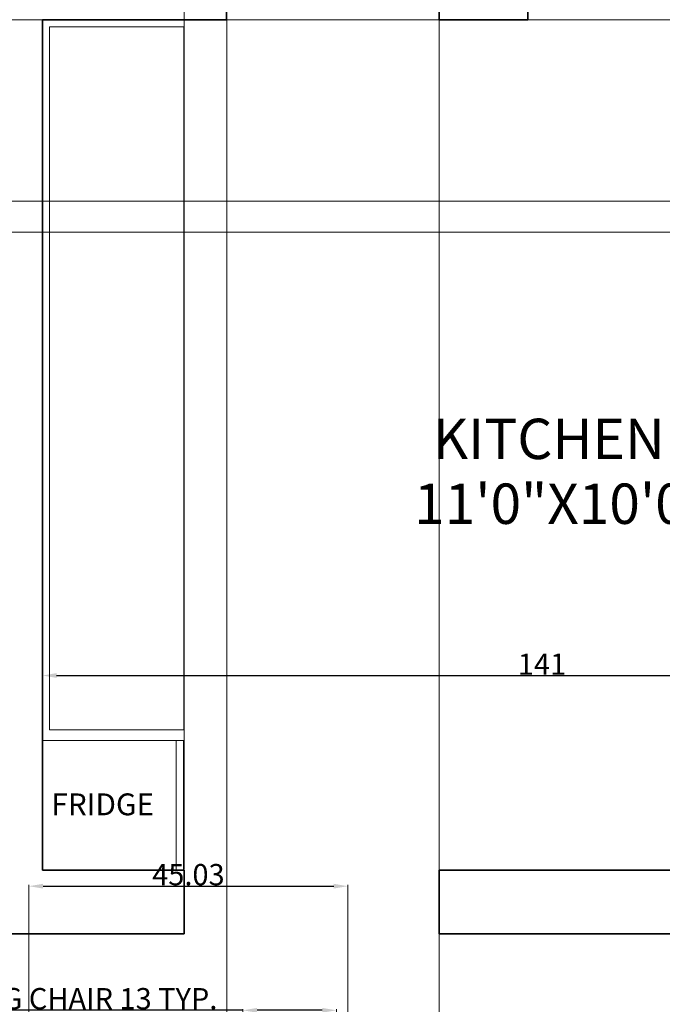
# Model space of a CAD drawing. Units: feet. Extents: x -297 to 770, y -228 to 625.
# Tile 8 of 14: x 589 to 680, y 95 to 233. Entities that reach past the tile are written whole.
import ezdxf

# ---------------------------------------------------------------- set-up
doc = ezdxf.new("R2010")
doc.units = ezdxf.units.FT
doc.header["$MEASUREMENT"] = 0
for name, color, linetype, lineweight in [('A-ANNO-DIMS', 2, 'Continuous', 18), ('A-ANNO-TEXT', 7, 'Continuous', 18), ('A-AREA-IDEN', 7, 'Continuous', 25), ('A-EQPM', 8, 'Continuous', 13), ('A-FLOR-CASE', 8, 'Continuous', 18), ('A-WALL', 7, 'Continuous', 35), ('doors', 30, 'Continuous', 18)]:
    doc.layers.add(name, color=color, linetype=linetype, lineweight=lineweight)
doc.styles.add('Annotative', font='arial.ttf')
doc.styles.get("Standard").update_dxf_attribs({"font": 'arial.ttf'})
doc.dimstyles.get("Standard").update_dxf_attribs({"dimtxt": 3, "dimasz": 2, "dimexe": 0.18, "dimexo": 0.0625, "dimgap": 0.09, "dimtad": 1, "dimtoh": 1, "dimdec": 1, "dimzin": 0, "dimdsep": 46, "dimlunit": 3, "dimtxsty": 'Standard', "dimcen": 0, "dimclre": 256, "dimadec": 0, "dimazin": 0, "dimtfac": 1, "dimtdec": 1, "dimtofl": 0, "dimtmove": 0, "dimatfit": 3, "dimfxl": 1, "dimtolj": 1, "dimtzin": 0, "dimlwe": -1, "dimarcsym": 0})

# ---------------------------------------------------------------- blocks, each defined once
blk = doc.blocks.new('*U6')
for p, q in [((0, 0), (0, -6)), ((40, 0), (40, -6))]:
    blk.add_line(p, q)
blk.add_lwpolyline([(0, 0), (0, 40), (1.75, 40), (1.75, 0)], close=True)
blk.add_arc((0, 0), 40, 0, 90)
blk = doc.blocks.new('*D23')
at = {"layer": 'A-ANNO-DIMS', "color": 0, "lineweight": -2, "transparency": 16777216}
for p, q in [((620.45, 93.67), (573.78, 93.67)), ((631.66, 93.67), (622.45, 93.67))]:
    blk.add_line(p, q, dxfattribs=at)
at = {"layer": 'A-ANNO-DIMS', "transparency": 16777216}
for p, q in [((620.45, 91.75), (620.45, 93.85)), ((633.66, 91.75), (633.66, 93.85))]:
    blk.add_line(p, q, dxfattribs=at)
at = {"layer": 'A-ANNO-DIMS', "color": 0, "transparency": 16777216}
for points in [[(622.45, 94), (622.45, 93.33), (620.45, 93.67)], [(631.66, 94), (631.66, 93.33), (633.66, 93.67)]]:
    blk.add_solid(points, dxfattribs=at)
at = {"layer": 'Defpoints', "color": 0, "transparency": 16777216}
for p in [(620.45, 93.67), (620.45, 91.69), (633.66, 91.69)]:
    blk.add_point(p, dxfattribs=at)
at = {"layer": 'A-ANNO-DIMS', "color": 0, "transparency": 16777216, "insert": (596.11, 95.31), "char_height": 3, "attachment_point": 5}
blk.add_mtext('\\A1;DINING CHAIR 13 TYP.', dxfattribs=at)
blk = doc.blocks.new('*D54')
at = {"layer": 'A-ANNO-DIMS', "transparency": 16777216}
for p, q in [((733.1, 233.46), (354.53, 233.46)), ((733.09, 203.46), (354.53, 203.46))]:
    blk.add_line(p, q, dxfattribs=at)
at = {"layer": 'A-ANNO-DIMS', "color": 0, "lineweight": -2, "transparency": 16777216}
blk.add_line((354.71, 205.46), (354.71, 231.46), dxfattribs=at)
at = {"layer": 'A-ANNO-DIMS', "color": 0, "transparency": 16777216}
for points in [[(354.37, 231.46), (355.04, 231.46), (354.71, 233.46)], [(354.37, 205.46), (355.04, 205.46), (354.71, 203.46)]]:
    blk.add_solid(points, dxfattribs=at)
at = {"layer": 'Defpoints', "color": 0, "transparency": 16777216}
for p in [(354.71, 233.46), (733.16, 233.46), (733.16, 203.46)]:
    blk.add_point(p, dxfattribs=at)
at = {"layer": 'A-ANNO-DIMS', "color": 0, "transparency": 16777216, "insert": (353.08, 218.46), "char_height": 3, "attachment_point": 5, "rotation": 90}
blk.add_mtext('\\A1;30', dxfattribs=at)
blk = doc.blocks.new('*D63')
at = {"layer": 'A-ANNO-DIMS', "transparency": 16777216}
for p, q in [((612.16, 113.53), (612.16, 367.22)), ((648.16, 113.53), (648.16, 367.22))]:
    blk.add_line(p, q, dxfattribs=at)
at = {"layer": 'A-ANNO-DIMS', "color": 0, "lineweight": -2, "transparency": 16777216}
blk.add_line((614.16, 367.04), (646.16, 367.04), dxfattribs=at)
at = {"layer": 'A-ANNO-DIMS', "color": 0, "transparency": 16777216}
for points in [[(614.16, 367.38), (614.16, 366.71), (612.16, 367.04)], [(646.16, 367.38), (646.16, 366.71), (648.16, 367.04)]]:
    blk.add_solid(points, dxfattribs=at)
at = {"layer": 'Defpoints', "color": 0, "transparency": 16777216}
for p in [(648.16, 367.04), (612.16, 113.46), (648.16, 113.46)]:
    blk.add_point(p, dxfattribs=at)
at = {"layer": 'A-ANNO-DIMS', "color": 0, "transparency": 16777216, "insert": (630.16, 368.66), "char_height": 3, "attachment_point": 5}
blk.add_mtext('\\A1;36', dxfattribs=at)
blk = doc.blocks.new('*D64')
at = {"layer": 'A-ANNO-DIMS', "transparency": 16777216}
for p, q in [((618.16, 233.4), (618.16, -227.67)), ((648.16, 233.4), (648.16, -227.67))]:
    blk.add_line(p, q, dxfattribs=at)
at = {"layer": 'A-ANNO-DIMS', "color": 0, "lineweight": -2, "transparency": 16777216}
blk.add_line((620.16, -227.49), (646.16, -227.49), dxfattribs=at)
at = {"layer": 'A-ANNO-DIMS', "color": 0, "transparency": 16777216}
for points in [[(620.16, -227.15), (620.16, -227.82), (618.16, -227.49)], [(646.16, -227.15), (646.16, -227.82), (648.16, -227.49)]]:
    blk.add_solid(points, dxfattribs=at)
at = {"layer": 'Defpoints', "color": 0, "transparency": 16777216}
for p in [(618.16, 233.46), (648.16, 233.46), (648.16, -227.49)]:
    blk.add_point(p, dxfattribs=at)
at = {"layer": 'A-ANNO-DIMS', "color": 0, "transparency": 16777216, "insert": (633.16, -225.86), "char_height": 3, "attachment_point": 5}
blk.add_mtext('\\A1;30', dxfattribs=at)
blk = doc.blocks.new('*D75')
at = {"layer": 'A-ANNO-DIMS', "transparency": 16777216}
for p, q in [((471.75, 264.96), (769.79, 264.96)), ((471.75, 207.87), (769.79, 207.87))]:
    blk.add_line(p, q, dxfattribs=at)
at = {"layer": 'A-ANNO-DIMS', "color": 0, "lineweight": -2, "transparency": 16777216}
blk.add_line((769.61, 209.87), (769.61, 262.96), dxfattribs=at)
at = {"layer": 'A-ANNO-DIMS', "color": 0, "transparency": 16777216}
for points in [[(769.27, 262.96), (769.94, 262.96), (769.61, 264.96)], [(769.27, 209.87), (769.94, 209.87), (769.61, 207.87)]]:
    blk.add_solid(points, dxfattribs=at)
at = {"layer": 'Defpoints', "color": 0, "transparency": 16777216}
for p in [(471.69, 264.96), (769.61, 264.96), (471.69, 207.87)]:
    blk.add_point(p, dxfattribs=at)
at = {"layer": 'A-ANNO-DIMS', "color": 0, "transparency": 16777216, "insert": (767.98, 236.42), "char_height": 3, "attachment_point": 5, "rotation": 90}
blk.add_mtext('\\A1;57.09', dxfattribs=at)
blk = doc.blocks.new('*D80')
at = {"layer": 'A-ANNO-DIMS', "transparency": 16777216}
for p, q in [((590.24, 83.79), (590.24, 111.36)), ((635.27, 83.79), (635.27, 111.36))]:
    blk.add_line(p, q, dxfattribs=at)
at = {"layer": 'A-ANNO-DIMS', "color": 0, "lineweight": -2, "transparency": 16777216}
blk.add_line((592.24, 111.18), (633.27, 111.18), dxfattribs=at)
at = {"layer": 'A-ANNO-DIMS', "color": 0, "transparency": 16777216}
for points in [[(592.24, 111.52), (592.24, 110.85), (590.24, 111.18)], [(633.27, 111.52), (633.27, 110.85), (635.27, 111.18)]]:
    blk.add_solid(points, dxfattribs=at)
at = {"layer": 'Defpoints', "color": 0, "transparency": 16777216}
for p in [(635.27, 111.18), (590.24, 83.73), (635.27, 83.73)]:
    blk.add_point(p, dxfattribs=at)
at = {"layer": 'A-ANNO-DIMS', "color": 0, "transparency": 16777216, "insert": (612.76, 112.81), "char_height": 3, "attachment_point": 5}
blk.add_mtext('\\A1;45.03', dxfattribs=at)
blk = doc.blocks.new('*D84')
at = {"layer": 'A-ANNO-DIMS', "transparency": 16777216}
for p, q in [((592.16, 113.53), (592.16, 141.09)), ((733.16, 113.53), (733.16, 141.09))]:
    blk.add_line(p, q, dxfattribs=at)
at = {"layer": 'A-ANNO-DIMS', "color": 0, "lineweight": -2, "transparency": 16777216}
blk.add_line((594.16, 140.91), (731.16, 140.91), dxfattribs=at)
at = {"layer": 'A-ANNO-DIMS', "color": 0, "transparency": 16777216}
for points in [[(594.16, 141.25), (594.16, 140.58), (592.16, 140.91)], [(731.16, 141.25), (731.16, 140.58), (733.16, 140.91)]]:
    blk.add_solid(points, dxfattribs=at)
at = {"layer": 'Defpoints', "color": 0, "transparency": 16777216}
for p in [(733.16, 140.91), (592.16, 113.46), (733.16, 113.46)]:
    blk.add_point(p, dxfattribs=at)
at = {"layer": 'A-ANNO-DIMS', "color": 0, "transparency": 16777216, "insert": (662.66, 142.51), "char_height": 3, "attachment_point": 5}
blk.add_mtext('\\A1;141', dxfattribs=at)

msp = doc.modelspace()

# ---------------------------------------------------------------- linework, layer by layer
at = {"layer": 'A-EQPM'}
msp.add_line((611.032, 113.463), (611.032, 131.761), dxfattribs=at)
msp.add_lwpolyline([(592.155, 113.463), (612.077, 113.463), (612.077, 131.761), (592.155, 131.761)], close=True, dxfattribs=at)
at = {"layer": 'A-FLOR-CASE'}
msp.add_lwpolyline([(593.155, 133.237), (612.118, 133.237), (612.118, 232.463), (593.155, 232.463)], close=True, dxfattribs=at)
at = {"layer": 'A-WALL'}
for p, q in [((618.155, 233.463), (618.155, 237.963)), ((648.155, 233.463), (648.155, 237.963)), ((660.655, 233.463), (660.655, 237.963)), ((592.155, 233.463), (592.155, 113.463)), ((618.155, 233.463), (592.155, 233.463)), ((660.655, 233.463), (648.155, 233.463)), ((592.155, 113.463), (612.155, 113.463)), ((612.155, 113.463), (612.155, 104.463)), ((733.155, 113.463), (648.155, 113.463)), ((648.155, 113.463), (648.155, 104.463)), ((587.655, 104.463), (612.155, 104.463)), ((733.155, 104.463), (648.155, 104.463))]:
    msp.add_line(p, q, dxfattribs=at)

# ---------------------------------------------------------------- block references
at = {"layer": 'doors', "xscale": 0.7226421799388985, "yscale": 0.7226421799388985, "zscale": 0.7226421799388985}
msp.add_blockref('*U6', (660.655, 237.799), dxfattribs=at)

# ---------------------------------------------------------------- texts
at = {"layer": 'A-ANNO-TEXT', "style": 'Annotative'}
msp.add_text('FRIDGE', height=3.0821, dxfattribs=at).set_placement((593.42, 121.191))
at = {"layer": 'A-AREA-IDEN', "style": 'Annotative'}
for s, height, p in [('KITCHEN', 5.696, (647.225, 171.459)), ('11\'0"X10\'0"', 5.69601, (644.619, 162.309))]:
    msp.add_text(s, height=height, dxfattribs=at).set_placement(p)

# ---------------------------------------------------------------- dimensions: what is measured, and where the dimension line sits
at = {"layer": 'A-ANNO-DIMS'}
for base, p1, p2, override, picture, middle in [((648.155, 367.042), (612.155, 113.463), (648.155, 113.463), {"dimdec": 0, "dimlfac": 1, "dimrnd": 0, "dimzin": 0, "dimdsep": 46, "dimlunit": 2}, '*D63', (630.155, 368.665)), ((648.155, -227.487), (618.155, 233.463), (648.155, 233.463), {"dimdec": 0, "dimlfac": 1, "dimrnd": 0, "dimzin": 0, "dimdsep": 46, "dimlunit": 2}, '*D64', (633.155, -225.865)), ((733.155, 140.913), (592.155, 113.463), (733.155, 113.463), {"dimdec": 0, "dimlfac": 1, "dimrnd": 0, "dimzin": 0, "dimdsep": 46, "dimlunit": 2}, '*D84', (662.655, 142.509)), ((635.271, 111.182), (590.239, 83.732), (635.271, 83.732), {"dimdec": 2, "dimlfac": 1, "dimrnd": 0, "dimzin": 0, "dimdsep": 46, "dimlunit": 2}, '*D80', (612.755, 112.805))]:
    dim = msp.add_linear_dim(base=base, p1=p1, p2=p2, dimstyle='Standard', override=override, dxfattribs=at)
    dim.commit()
    dim.dimension.update_dxf_attribs({"geometry": picture, "text_midpoint": middle})
for base, p1, p2, override, picture, middle in [((769.605, 264.961), (471.691, 207.869), (471.691, 264.961), {"dimdec": 2, "dimlfac": 1, "dimrnd": 0, "dimzin": 0, "dimdsep": 46, "dimlunit": 2}, '*D75', (767.984, 236.415)), ((354.705, 233.463), (733.155, 203.463), (733.158, 233.463), {"dimdec": 0, "dimlfac": 1, "dimrnd": 0, "dimzin": 0, "dimdsep": 46, "dimlunit": 2}, '*D54', (353.083, 218.463))]:
    dim = msp.add_linear_dim(base=base, p1=p1, p2=p2, angle=90, dimstyle='Standard', override=override, dxfattribs=at)
    dim.commit()
    dim.dimension.update_dxf_attribs({"geometry": picture, "text_midpoint": middle})
dim = msp.add_linear_dim(base=(620.45, 93.666), p1=(633.656, 91.685), p2=(620.45, 91.685), angle=180, text='DINING CHAIR <> TYP.', dimstyle='Standard', override={"dimdec": 0, "dimlfac": 1, "dimrnd": 0, "dimzin": 0, "dimdsep": 46, "dimlunit": 2}, dxfattribs=at)
dim.commit()
dim.dimension.update_dxf_attribs({"geometry": '*D23', "text_midpoint": (596.115, 95.309)})

doc.saveas('drawing.dxf')
